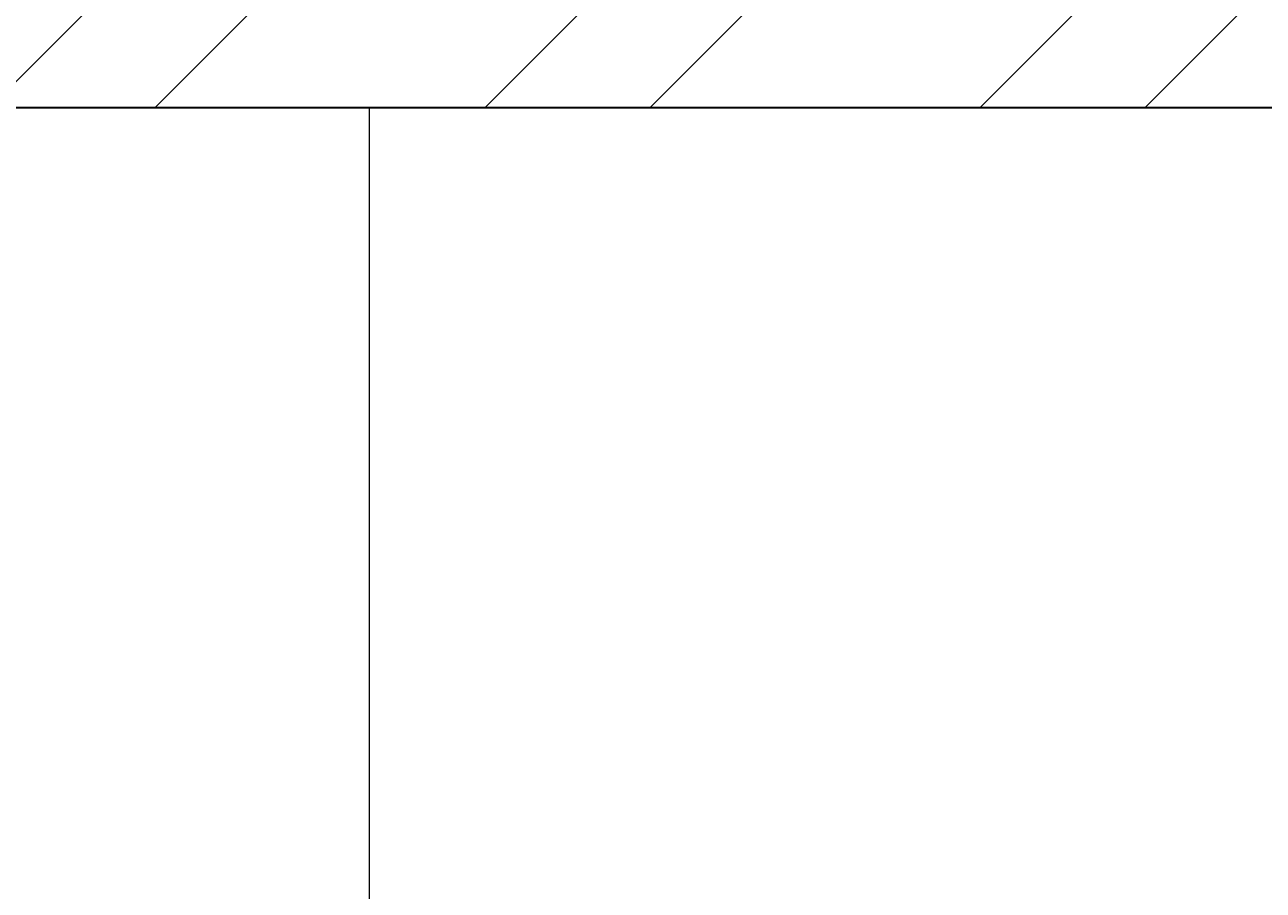
# Model space of a CAD drawing. Units: inches. Extents: x 1885 to 2748, y 783 to 2421.
# Tile 78 of 117: x 2004 to 2038, y 2144 to 2167. Entities that reach past the tile are written whole.
import ezdxf

# ---------------------------------------------------------------- set-up
doc = ezdxf.new("R2010")
doc.units = ezdxf.units.IN
for name, color, linetype, lineweight in [('A-ANNO-DIMS', 2, 'Continuous', 18), ('A-FLOR-CASE', 9, 'Continuous', 18), ('A-WALL', 7, 'Continuous', 35)]:
    doc.layers.add(name, color=color, linetype=linetype, lineweight=lineweight)
doc.layers.add('A-WALL-PATT', color=85, linetype='Continuous', lineweight=13, true_color=0x58ba48)
doc.styles.get("Standard").update_dxf_attribs({"font": 'arial.ttf'})
doc.dimstyles.get("Standard").update_dxf_attribs({"dimtxt": 0.18, "dimasz": 0.18, "dimexe": 0.18, "dimexo": 0.0625, "dimgap": 0.09, "dimtad": 0, "dimtih": 1, "dimtoh": 1, "dimdec": 4, "dimzin": 0, "dimdsep": 46, "dimtxsty": 'Standard', "dimcen": 0.09, "dimadec": 0, "dimazin": 0, "dimtfac": 1, "dimtdec": 4, "dimtofl": 0, "dimtmove": 0, "dimatfit": 3, "dimfxl": 1, "dimtolj": 1, "dimtzin": 0, "dimarcsym": 0})

# ---------------------------------------------------------------- blocks, each defined once
blk = doc.blocks.new('*D48')
at = {"layer": 'A-ANNO-DIMS', "color": 0, "lineweight": -2, "transparency": 16777216}
for p, q in [((1980.711, 2348.006), (1902.844, 2348.006)), ((1903.024, 2347.826), (1903.024, 2114.937)), ((1903.024, 1881.686), (1903.024, 2114.574)), ((2016.711, 1881.506), (1902.844, 1881.506))]:
    blk.add_line(p, q, dxfattribs=at)
at = {"layer": 'A-ANNO-DIMS', "color": 0, "transparency": 16777216}
for points in [[(1902.994, 2347.826), (1903.054, 2347.826), (1903.024, 2348.006)], [(1902.994, 1881.686), (1903.054, 1881.686), (1903.024, 1881.506)]]:
    blk.add_solid(points, dxfattribs=at)
at = {"layer": 'Defpoints', "color": 0, "transparency": 16777216}
for p in [(1903.024, 2348.006), (1980.774, 2348.006), (2016.774, 1881.506)]:
    blk.add_point(p, dxfattribs=at)
at = {"layer": 'A-ANNO-DIMS', "color": 0, "transparency": 16777216, "insert": (1903.024, 2114.756), "char_height": 0.18, "attachment_point": 5}
blk.add_mtext('\\A1;466.5', dxfattribs=at)

msp = doc.modelspace()

# ---------------------------------------------------------------- hatches: boundary and pattern name
at = {"layer": 'A-WALL-PATT'}
h = msp.add_hatch(dxfattribs=at)
h.set_pattern_fill('ANSI32', color=256)
h.paths.add_polyline_path([(2007.772, 2318.006), (1980.774, 2318.006), (1980.774, 2281.215), (1985.274, 2281.215), (1985.274, 2313.506), (2007.772, 2313.506), (2007.772, 2315.756)])
h.paths.add_polyline_path([(2094.324, 2318.006), (2067.772, 2318.006), (2067.772, 2313.506), (2094.324, 2313.506), (2094.324, 2315.756)])
h.paths.add_polyline_path([(2131.367, 2315.756), (2131.367, 2318.006), (2131.189, 2318.006), (2112.609, 2318.006), (2112.609, 2313.506), (2117.274, 2313.506), (2117.274, 2255.201), (2121.774, 2255.201), (2121.774, 2313.506), (2131.367, 2313.506)])
h.paths.add_polyline_path([(2190.512, 2318.006), (2155.367, 2318.006), (2155.367, 2313.506), (2169.774, 2313.506), (2169.774, 2229.506), (2121.774, 2229.506), (2121.774, 2233.451), (2119.524, 2233.451), (2117.274, 2233.451), (2117.274, 2201.101), (2121.774, 2201.101), (2121.774, 2225.006), (2169.774, 2225.006), (2169.774, 2165.006), (2306.274, 2165.006), (2306.274, 2066.006), (2310.774, 2066.006), (2344.274, 2066.006), (2486.274, 2066.006), (2486.274, 1886.006), (2483.02, 1886.006), (2483.02, 1881.506), (2486.274, 1881.506), (2486.274, 1880.678), (2490.774, 1880.678), (2490.774, 2070.506), (2344.274, 2070.506), (2310.774, 2070.506), (2310.774, 2165.006), (2310.774, 2173.636), (2308.524, 2173.636), (2306.274, 2173.636), (2306.274, 2169.506), (2174.274, 2169.506), (2174.274, 2313.506), (2190.512, 2313.506), (2190.512, 2315.756)])
h.paths.add_polyline_path([(1985.274, 2221.215), (1980.774, 2221.215), (1980.774, 2165.006), (1992.774, 2165.006), (1992.774, 2141.927), (1997.274, 2141.927), (1997.274, 2165.006), (2117.274, 2165.006), (2117.274, 2163.126), (2121.774, 2163.126), (2121.774, 2172.734), (2119.524, 2172.734), (2117.274, 2172.734), (2117.274, 2169.506), (1985.274, 2169.506)])
h.paths.add_polyline_path([(1997.274, 2105.927), (1992.774, 2105.927), (1992.774, 2070.506), (2016.774, 2070.506), (2016.774, 2059.123), (2019.024, 2059.123), (2021.274, 2059.123), (2021.274, 2070.506), (2117.274, 2070.506), (2117.274, 2022.506), (2114.423, 2022.506), (2114.423, 2018.006), (2123.627, 2018.006), (2123.627, 2020.256), (2123.627, 2022.506), (2121.774, 2022.506), (2121.774, 2142.587), (2119.524, 2142.587), (2117.274, 2142.587), (2117.274, 2075.006), (1997.274, 2075.006)])
h.paths.add_polyline_path([(2092.029, 2020.256), (2092.029, 2022.506), (2021.274, 2022.506), (2021.274, 2035.123), (2016.774, 2035.123), (2016.774, 2018.006), (2016.774, 1978.784), (2021.274, 1978.784), (2021.274, 2018.006), (2092.029, 2018.006)])
h.paths.add_polyline_path([(2260.938, 2022.506), (2153.105, 2022.506), (2153.105, 2020.256), (2153.105, 2018.006), (2155.274, 2018.006), (2155.274, 1886.006), (2107.629, 1886.006), (2107.629, 1881.506), (2182.911, 1881.506), (2182.911, 1883.756), (2182.911, 1886.006), (2159.774, 1886.006), (2159.774, 2018.006), (2260.938, 2018.006), (2260.938, 2020.256)])
h.paths.add_polyline_path([(2047.629, 1883.756), (2047.629, 1886.006), (2021.274, 1886.006), (2021.274, 1918.784), (2019.024, 1918.784), (2016.774, 1918.784), (2016.774, 1881.506), (2047.629, 1881.506)])
h.paths.add_polyline_path([(2306.361, 1883.756), (2306.361, 1886.006), (2296.274, 1886.006), (2296.274, 1982.006), (2316.535, 1982.006), (2316.535, 1984.256), (2316.535, 1986.506), (2296.274, 1986.506), (2296.274, 2022.506), (2289.276, 2022.506), (2289.276, 2018.006), (2291.774, 2018.006), (2291.774, 1886.006), (2242.911, 1886.006), (2242.911, 1881.506), (2306.361, 1881.506)], flags=17)
h.paths.add_polyline_path([(1985.274, 1843.006), (2021.6, 1843.006), (2021.534, 1845.441), (2021.477, 1847.506), (1980.774, 1847.506), (1980.774, 1809.446), (1985.274, 1809.446)])
h.paths.add_polyline_path([(2131.482, 1845.256), (2131.482, 1847.506), (2081.534, 1847.506), (2081.534, 1843.006), (2117.274, 1843.006), (2117.274, 1784.147), (2119.524, 1784.147), (2121.774, 1784.147), (2121.774, 1843.006), (2131.482, 1843.006)])
h.paths.add_polyline_path([(2203.886, 1847.506), (2155.482, 1847.506), (2155.482, 1843.006), (2169.774, 1843.006), (2169.774, 1759.006), (2121.774, 1759.006), (2121.774, 1761.457), (2117.274, 1761.457), (2117.274, 1730.429), (2121.774, 1730.429), (2121.774, 1754.506), (2177.421, 1754.506), (2177.421, 1756.756), (2177.421, 1759.006), (2174.274, 1759.006), (2174.274, 1843.006), (2203.886, 1843.006)])
h.paths.add_polyline_path([(2335.554, 1845.256), (2335.554, 1847.506), (2239.886, 1847.506), (2239.886, 1843.006), (2306.274, 1843.006), (2306.274, 1759.006), (2199.486, 1759.006), (2199.486, 1754.506), (2310.774, 1754.506), (2310.774, 1843.006), (2335.554, 1843.006)])
h.paths.add_polyline_path([(2348.774, 2022.506), (2344.274, 2022.506), (2344.274, 1986.506), (2341.681, 1986.506), (2341.681, 1982.006), (2344.274, 1982.006), (2344.274, 1886.006), (2330.361, 1886.006), (2330.361, 1881.506), (2361.627, 1881.506), (2361.627, 1883.756), (2361.627, 1886.006), (2348.774, 1886.006)], flags=17)
h.paths.add_polyline_path([(2283.251, 2315.756), (2283.251, 2318.006), (2238.512, 2318.006), (2238.512, 2313.506), (2283.251, 2313.506)], flags=17)
h.paths.add_polyline_path([(2363.274, 2348.006), (2388.677, 2348.006), (2388.677, 2350.256), (2388.677, 2352.506), (2358.774, 2352.506), (2358.774, 2348.006), (2358.774, 2318.006), (2344.481, 2318.006), (2344.481, 2313.506), (2358.774, 2313.506), (2358.774, 2229.506), (2310.774, 2229.506), (2310.774, 2231.952), (2306.274, 2231.952), (2306.274, 2205.611), (2310.774, 2205.611), (2310.774, 2225.006), (2358.774, 2225.006), (2358.774, 2211.506), (2452.329, 2211.506), (2452.329, 2213.756), (2452.329, 2216.006), (2363.274, 2216.006), (2363.274, 2318.006)])
h.paths.add_polyline_path([(2310.774, 2313.506), (2320.481, 2313.506), (2320.481, 2315.756), (2320.481, 2318.006), (2302.728, 2318.006), (2302.728, 2313.506), (2306.274, 2313.506), (2306.274, 2251.076), (2310.774, 2251.076)], flags=17)
h.paths.add_polyline_path([(2490.774, 2352.506), (2486.274, 2352.506), (2448.677, 2352.506), (2448.677, 2348.006), (2486.274, 2348.006), (2486.274, 2318.006), (2486.274, 2216.006), (2481.78, 2216.006), (2481.78, 2211.506), (2486.274, 2211.506), (2486.274, 2165.006), (2493.289, 2165.006), (2493.289, 2167.256), (2493.289, 2169.506), (2490.774, 2169.506), (2490.774, 2313.506), (2494.429, 2313.506), (2494.429, 2318.006), (2490.774, 2318.006)])
h.paths.add_polyline_path([(2534.653, 2318.006), (2515.691, 2318.006), (2515.691, 2313.506), (2534.653, 2313.506), (2534.653, 2315.756)])
h.paths.add_polyline_path([(2618.274, 2318.006), (2594.653, 2318.006), (2594.653, 2313.506), (2613.774, 2313.506), (2613.774, 2281.706), (2618.274, 2281.706)])
h.paths.add_polyline_path([(2618.274, 2221.706), (2613.774, 2221.706), (2613.774, 2169.506), (2554.019, 2169.506), (2554.019, 2165.006), (2613.774, 2165.006), (2613.774, 2152.878), (2618.274, 2152.878)])
h.paths.add_polyline_path([(2618.274, 2128.878), (2616.024, 2128.878), (2613.774, 2128.878), (2613.774, 2117.006), (2529.774, 2117.006), (2529.774, 2165.006), (2532.848, 2165.006), (2532.848, 2169.506), (2522.867, 2169.506), (2522.867, 2165.006), (2525.274, 2165.006), (2525.274, 2117.006), (2525.274, 2112.506), (2525.274, 2108.576), (2529.774, 2108.576), (2529.774, 2112.506), (2613.774, 2112.506), (2613.774, 2080.19), (2618.274, 2080.19)])
h.paths.add_polyline_path([(2618.274, 2044.19), (2616.024, 2044.19), (2613.774, 2044.19), (2613.774, 2015.506), (2529.774, 2015.506), (2529.774, 2088.582), (2527.524, 2088.582), (2525.274, 2088.582), (2525.274, 2011.006), (2613.774, 2011.006), (2613.774, 1956.755), (2618.274, 1956.755)])
h.paths.add_polyline_path([(2618.274, 1881.506), (2618.274, 1896.755), (2613.774, 1896.755), (2613.774, 1881.506), (2613.774, 1847.506), (2592.715, 1847.506), (2592.715, 1843.006), (2613.774, 1843.006), (2613.774, 1765.006), (2613.774, 1760.506), (2609.621, 1760.506), (2609.621, 1756.006), (2613.774, 1756.006), (2613.774, 1660.006), (2608.544, 1660.006), (2608.544, 1655.506), (2613.774, 1655.506), (2613.774, 1508.158), (2618.274, 1508.158)])
h.paths.add_polyline_path([(2565.774, 1843.006), (2568.997, 1843.006), (2568.997, 1847.506), (2490.774, 1847.506), (2490.774, 1849.7), (2488.524, 1849.7), (2486.274, 1849.7), (2486.274, 1847.506), (2477.274, 1847.506), (2477.274, 1838.506), (2477.274, 1821.493), (2486.274, 1821.493), (2486.274, 1838.506), (2561.274, 1838.506), (2561.274, 1765.006), (2486.274, 1765.006), (2486.274, 1786.157), (2477.274, 1786.157), (2477.274, 1765.006), (2477.274, 1756.006), (2486.274, 1756.006), (2565.774, 1756.006), (2585.621, 1756.006), (2585.621, 1758.256), (2585.621, 1760.506), (2565.774, 1760.506), (2565.774, 1765.006)])
h.paths.add_polyline_path([(2486.274, 1651.006), (2561.274, 1651.006), (2561.274, 1567.006), (2486.274, 1567.006), (2486.274, 1591.321), (2477.274, 1591.321), (2477.274, 1567.006), (2477.274, 1558.006), (2477.274, 1555.439), (2481.774, 1555.439), (2481.774, 1558.006), (2568.653, 1558.006), (2568.653, 1560.256), (2568.653, 1562.506), (2565.774, 1562.506), (2565.774, 1655.506), (2584.544, 1655.506), (2584.544, 1657.756), (2584.544, 1660.006), (2565.774, 1660.006), (2486.274, 1660.006), (2477.274, 1660.006), (2477.274, 1651.006), (2477.274, 1632.989), (2486.274, 1632.989)])
h.paths.add_polyline_path([(2449.967, 1883.756), (2449.967, 1886.006), (2421.627, 1886.006), (2421.627, 1881.506), (2449.967, 1881.506)], flags=17)
h.paths.add_polyline_path([(2447.274, 1847.506), (2395.554, 1847.506), (2395.554, 1843.006), (2442.774, 1843.006), (2442.774, 1809.27), (2447.274, 1809.27)])
h.paths.add_polyline_path([(1985.274, 1749.446), (1980.774, 1749.446), (1980.774, 1694.504), (1985.274, 1694.504), (1985.274, 1694.506), (1986.897, 1694.506), (1986.897, 1697.78), (1986.897, 1699.006), (1985.274, 1699.006)])
h.paths.add_polyline_path([(2152.774, 1699.006), (2121.774, 1699.006), (2121.774, 1703.668), (2119.524, 1703.668), (2117.274, 1703.668), (2117.274, 1699.006), (2009.219, 1699.006), (2009.219, 1694.506), (2148.274, 1694.506), (2148.274, 1692.631), (2152.774, 1692.631)])
h.paths.add_polyline_path([(2016.274, 1694.506), (2011.774, 1694.506), (2011.774, 1558.006), (2040.806, 1558.006), (2040.806, 1560.256), (2040.806, 1562.506), (2016.274, 1562.506)])
h.paths.add_polyline_path([(2152.774, 1663.017), (2150.524, 1663.017), (2148.274, 1663.017), (2148.274, 1562.506), (2100.806, 1562.506), (2100.806, 1558.006), (2165.119, 1558.006), (2165.119, 1560.256), (2165.119, 1562.506), (2152.774, 1562.506), (2152.774, 1610.506), (2224.774, 1610.506), (2224.774, 1607.99), (2229.274, 1607.99), (2229.274, 1615.006), (2152.774, 1615.006)])
h.paths.add_polyline_path([(2238.613, 1560.256), (2238.613, 1562.506), (2229.274, 1562.506), (2229.274, 1588.756), (2227.024, 1588.763), (2224.774, 1588.771), (2224.774, 1562.506), (2189.119, 1562.506), (2189.119, 1558.006), (2238.613, 1558.006)])
h.paths.add_polyline_path([(2336.024, 1560.256), (2336.024, 1562.506), (2310.774, 1562.506), (2310.774, 1656.347), (2308.524, 1656.347), (2306.274, 1656.347), (2306.274, 1562.506), (2286.613, 1562.506), (2286.613, 1558.006), (2336.024, 1558.006)])
h.paths.add_polyline_path([(2447.274, 1690.968), (2445.024, 1690.968), (2442.774, 1690.968), (2442.774, 1687.006), (2306.274, 1687.006), (2306.274, 1680.75), (2310.774, 1680.75), (2310.774, 1682.506), (2442.774, 1682.506), (2442.774, 1562.506), (2396.024, 1562.506), (2396.024, 1558.006), (2447.274, 1558.006)])
h.paths.add_polyline_path([(2447.274, 1749.27), (2445.024, 1749.27), (2442.774, 1749.27), (2442.774, 1717.232), (2447.274, 1717.232)])
h.paths.add_polyline_path([(2044.674, 1521.756), (2044.674, 1524.006), (2007.274, 1524.006), (2007.274, 1503.49), (2009.524, 1503.49), (2011.774, 1503.49), (2011.774, 1519.506), (2044.674, 1519.506)])
h.paths.add_polyline_path([(2177.969, 1521.756), (2177.969, 1524.006), (2104.674, 1524.006), (2104.674, 1519.506), (2145.774, 1519.506), (2145.774, 1387.506), (2143.37, 1387.506), (2143.37, 1383.006), (2251.585, 1383.006), (2251.585, 1385.256), (2251.585, 1387.506), (2150.274, 1387.506), (2150.274, 1519.506), (2177.969, 1519.506)])
h.paths.add_polyline_path([(2298.704, 1524.006), (2237.969, 1524.006), (2237.969, 1519.506), (2282.274, 1519.506), (2282.274, 1387.506), (2279.683, 1387.506), (2279.683, 1383.006), (2286.774, 1383.006), (2286.774, 1419.006), (2312.451, 1419.006), (2312.451, 1421.256), (2312.451, 1423.506), (2286.774, 1423.506), (2286.774, 1519.506), (2298.704, 1519.506), (2298.704, 1521.722)], flags=17)
h.paths.add_polyline_path([(2361.897, 1521.756), (2361.897, 1524.006), (2322.704, 1524.006), (2322.704, 1519.506), (2334.774, 1519.506), (2334.774, 1423.506), (2331.93, 1423.506), (2331.93, 1419.006), (2334.774, 1419.006), (2334.774, 1387.506), (2334.774, 1383.228), (2339.274, 1383.228), (2339.274, 1387.506), (2339.274, 1519.506), (2361.897, 1519.506)], flags=17)
h.paths.add_polyline_path([(2447.274, 1521.756), (2447.274, 1524.006), (2421.897, 1524.006), (2421.897, 1519.506), (2447.274, 1519.506)], flags=17)
h.paths.add_polyline_path([(2481.774, 1529.6), (2479.524, 1529.6), (2477.274, 1529.6), (2477.274, 1524.006), (2474.489, 1524.006), (2474.489, 1519.506), (2477.274, 1519.506), (2477.274, 1334.506), (2296.774, 1334.506), (2296.774, 1240.506), (2160.274, 1240.506), (2160.274, 1180.506), (2112.274, 1180.506), (2112.274, 1207.692), (2110.024, 1207.692), (2107.774, 1207.692), (2107.774, 1171.609), (2112.274, 1171.609), (2112.274, 1176.006), (2160.274, 1176.006), (2160.274, 1092.006), (2144.221, 1092.006), (2144.221, 1087.506), (2189.497, 1087.506), (2189.497, 1089.756), (2189.497, 1092.006), (2164.774, 1092.006), (2164.774, 1236.006), (2296.774, 1236.006), (2296.774, 1231.912), (2301.274, 1231.912), (2301.274, 1330.006), (2481.774, 1330.006), (2481.774, 1387.506)])
h.paths.add_polyline_path([(2618.274, 1448.158), (2613.774, 1448.158), (2613.774, 1382.506), (2529.774, 1382.506), (2525.274, 1382.506), (2525.274, 1307.062), (2529.774, 1307.062), (2529.774, 1378.006), (2613.774, 1378.006), (2613.774, 1354.988), (2618.274, 1354.988)])
h.paths.add_polyline_path([(2618.274, 1318.988), (2613.774, 1318.988), (2613.774, 1281.006), (2529.774, 1281.006), (2529.774, 1283.786), (2527.524, 1283.786), (2525.274, 1283.786), (2525.274, 1228.506), (2516.794, 1228.506), (2516.794, 1224.006), (2533.484, 1224.006), (2533.484, 1226.256), (2533.484, 1228.506), (2529.774, 1228.506), (2529.774, 1276.506), (2613.774, 1276.506), (2613.774, 1266.02), (2618.274, 1266.02)])
h.paths.add_polyline_path([(2618.274, 1134.964), (2613.774, 1134.964), (2613.774, 1092.006), (2594.545, 1092.006), (2594.545, 1087.506), (2618.274, 1087.506)])
h.paths.add_polyline_path([(2534.545, 1092.006), (2509.765, 1092.006), (2509.765, 1087.506), (2534.545, 1087.506), (2534.545, 1089.756)])
h.paths.add_polyline_path([(2481.274, 1224.006), (2484.117, 1224.006), (2484.117, 1226.256), (2484.117, 1228.506), (2476.774, 1228.506), (2476.774, 1198.506), (2471.61, 1198.506), (2471.61, 1194.006), (2476.774, 1194.006), (2476.774, 1062.006), (2436.894, 1062.006), (2436.894, 1057.506), (2476.774, 1057.506), (2481.274, 1057.506), (2481.274, 1062.006), (2481.274, 1087.506), (2485.354, 1087.506), (2485.354, 1089.756), (2485.354, 1092.006), (2481.274, 1092.006), (2481.274, 1117.506)])
h.paths.add_polyline_path([(2439.898, 1198.506), (2349.274, 1198.506), (2349.274, 1194.006), (2349.274, 1180.506), (2301.274, 1180.506), (2301.274, 1201.896), (2299.024, 1201.896), (2296.774, 1201.896), (2296.774, 1172.335), (2299.024, 1172.335), (2301.274, 1172.335), (2301.274, 1176.006), (2349.274, 1176.006), (2349.274, 1092.006), (2334.452, 1092.006), (2334.452, 1087.506), (2349.274, 1087.506), (2349.274, 1057.506), (2353.774, 1057.506), (2376.894, 1057.506), (2376.894, 1059.756), (2376.894, 1062.006), (2353.774, 1062.006), (2353.774, 1087.506), (2353.774, 1180.506), (2353.774, 1194.006), (2439.898, 1194.006), (2439.898, 1196.256)])
h.paths.add_polyline_path([(2270.596, 1089.756), (2270.596, 1092.006), (2249.497, 1092.006), (2249.497, 1087.506), (2270.596, 1087.506)], flags=17)
h.paths.add_polyline_path([(2310.452, 1092.006), (2301.274, 1092.006), (2301.274, 1153.292), (2296.774, 1153.292), (2296.774, 1092.006), (2293.786, 1092.006), (2293.786, 1087.506), (2310.452, 1087.506), (2310.452, 1089.756)], flags=17)
h.paths.add_polyline_path([(2112.274, 1150.328), (2110.024, 1150.328), (2107.774, 1150.328), (2107.774, 1092.006), (2104.465, 1092.006), (2104.465, 1087.506), (2120.221, 1087.506), (2120.221, 1089.756), (2120.221, 1092.006), (2112.274, 1092.006)])
h.paths.add_polyline_path([(2082.172, 1092.006), (2058.144, 1092.006), (2058.144, 1087.506), (2082.172, 1087.506), (2082.172, 1089.756)])
h.paths.add_polyline_path([(1975.774, 1145.638), (1971.274, 1145.638), (1971.274, 1087.506), (1980.774, 1087.506), (1998.144, 1087.506), (1998.144, 1089.756), (1998.144, 1092.006), (1985.274, 1092.006), (1975.774, 1092.006)])
h.paths.add_polyline_path([(2112.274, 1244.385), (2110.024, 1244.385), (2107.774, 1244.385), (2107.774, 1240.506), (1992.274, 1240.506), (1992.274, 1271.008), (1987.774, 1271.008), (1987.774, 1240.506), (1980.774, 1240.506), (1975.774, 1240.506), (1971.274, 1240.506), (1971.274, 1205.638), (1975.774, 1205.638), (1975.774, 1236.006), (2107.774, 1236.006), (2107.774, 1233.444), (2112.274, 1233.444), (2112.274, 1236.006)])
h.paths.add_polyline_path([(2112.274, 1383.006), (2114.783, 1383.006), (2114.783, 1385.256), (2114.783, 1387.506), (2102.476, 1387.506), (2102.476, 1383.006), (2107.774, 1383.006), (2107.774, 1335.006), (2011.774, 1335.006), (2011.774, 1349.939), (2007.274, 1349.939), (2007.274, 1335.006), (1987.774, 1335.006), (1987.774, 1330.506), (1987.774, 1307.008), (1992.274, 1307.008), (1992.274, 1330.506), (2007.274, 1330.506), (2107.774, 1330.506), (2107.774, 1264.711), (2112.274, 1264.711)])
h.paths.add_polyline_path([(2077.857, 1387.506), (2011.774, 1387.506), (2011.774, 1390.036), (2009.524, 1390.036), (2007.274, 1390.036), (2007.274, 1373.939), (2011.774, 1373.939), (2011.774, 1383.006), (2077.857, 1383.006)])
h.paths.add_polyline_path([(2011.774, 1443.49), (2007.274, 1443.49), (2007.274, 1410.248), (2011.774, 1410.248)])

# ---------------------------------------------------------------- linework, layer by layer
at = {"layer": 'A-FLOR-CASE'}
msp.add_line((2013.676, 2165.006), (2013.676, 2093.221), dxfattribs=at)
at = {"layer": 'A-WALL'}
msp.add_line((1997.274, 2165.006), (2117.274, 2165.006), dxfattribs=at)

# ---------------------------------------------------------------- dimensions: what is measured, and where the dimension line sits
at = {"layer": 'A-ANNO-DIMS'}
dim = msp.add_linear_dim(base=(1903.024, 2348.006), p1=(2016.774, 1881.506), p2=(1980.774, 2348.006), angle=90, dimstyle='Standard', override={"dimdec": 1, "dimlfac": 1, "dimrnd": 0, "dimzin": 0, "dimdsep": 46, "dimlunit": 2}, dxfattribs=at)
dim.commit()
dim.dimension.update_dxf_attribs({"geometry": '*D48', "text_midpoint": (1903.024, 2114.756)})

doc.saveas('drawing.dxf')
